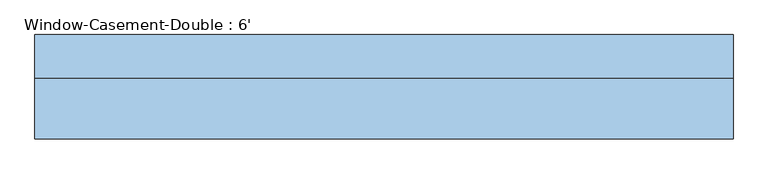
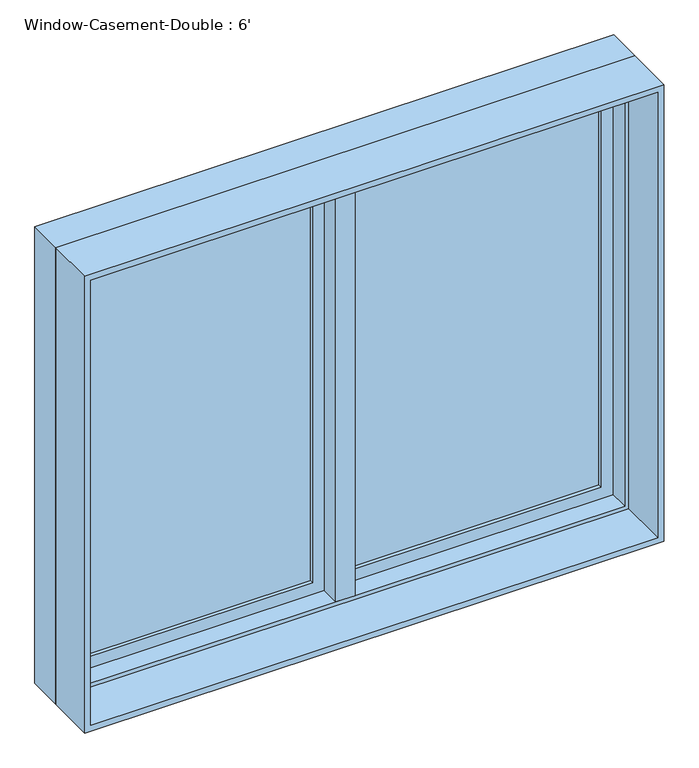
"""IFC4 building model written with IfcOpenShell, lengths in millimetres: window geometry, Window-Casement-Double : 6'."""

from ifc_helpers import new_model, si_unit, frame, origin, place, context, project, spatial, polyline, outline, extrude, faceted_brep, source, transform, mapped, element, save


def window_casement_double_6_75db422f(model_context):
    return source(origin(), model_context, "Body", "SolidModel", [
        faceted_brep([(9.525, 146.05, 2425.7), (-9.525, 146.05, 2425.7), (-9.525, 95.25, 2425.7), (9.525, 95.25, 2425.7), (9.525, 146.05, 927.1), (9.525, 95.25, 927.1), (-9.525, 95.25, 927.1), (-9.525, 146.05, 927.1), (-9.525, 95.25, 946.15), (-9.525, 95.25, 2406.65), (-30.1625, 95.25, 946.15), (-30.1625, 95.25, 2406.65), (-30.1625, 31.75, 946.15), (-30.1625, 31.75, 2406.65), (30.1625, 31.75, 946.15), (30.1625, 31.75, 2406.65), (30.1625, 95.25, 946.15), (30.1625, 95.25, 2406.65), (9.525, 95.25, 946.15), (9.525, 95.25, 2406.65)], [[[0, 1, 2, 3]], [[4, 5, 6, 7]], [[1, 0, 4, 7]], [[2, 1, 7, 6, 8, 9]], [[9, 8, 10, 11]], [[11, 10, 12, 13]], [[13, 12, 14, 15]], [[15, 14, 16, 17]], [[17, 16, 18, 19]], [[0, 3, 19, 18, 5, 4]], [[18, 8, 6, 5]], [[9, 19, 3, 2]], [[8, 18, 16, 14, 12, 10]], [[19, 9, 11, 13, 15, 17]]]),
        extrude(outline(polyline([(-66.675, 127.0), (-66.675, 120.65), (-844.55, 120.65), (-844.55, 127.0), (-66.675, 127.0)])), frame((0.0, 0.0, 984.25), z_axis=(0.0, 0.0, 1.0), x_axis=(1.0, 0.0, 0.0)), (0.0, 0.0, 1.0), 1384.3),
        extrude(outline(polyline([(-844.55, 107.95), (-844.55, 114.3), (-66.675, 114.3), (-66.675, 107.95), (-844.55, 107.95)])), frame((0.0, 0.0, 984.25), z_axis=(0.0, 0.0, 1.0), x_axis=(1.0, 0.0, 0.0)), (0.0, 0.0, 1.0), 1384.3),
        extrude(outline(polyline([(844.55, 127.0), (844.55, 120.65), (66.675, 120.65), (66.675, 127.0), (844.55, 127.0)])), frame((0.0, 0.0, 984.25), z_axis=(0.0, 0.0, 1.0), x_axis=(1.0, 0.0, 0.0)), (0.0, 0.0, 1.0), 1384.3),
        extrude(outline(polyline([(66.675, 107.95), (66.675, 114.3), (844.55, 114.3), (844.55, 107.95), (66.675, 107.95)])), frame((0.0, 0.0, 984.25), z_axis=(0.0, 0.0, 1.0), x_axis=(1.0, 0.0, 0.0)), (0.0, 0.0, 1.0), 1384.3),
        extrude(outline(polyline([(2425.7, -901.7), (927.1, -901.7), (927.1, -9.525), (2425.7, -9.525), (2425.7, -901.7)]), holes=[polyline([(2368.55, -66.675), (984.25, -66.675), (984.25, -844.55), (2368.55, -844.55), (2368.55, -66.675)])]), frame((0.0, 95.25, 0.0), z_axis=(0.0, 1.0, 0.0), x_axis=(0.0, 0.0, 1.0)), (0.0, 0.0, 1.0), 44.45),
        extrude(outline(polyline([(927.1, 901.7), (2425.7, 901.7), (2425.7, 9.525), (927.1, 9.525), (927.1, 901.7)]), holes=[polyline([(984.25, 66.675), (2368.55, 66.675), (2368.55, 844.55), (984.25, 844.55), (984.25, 66.675)])]), frame((0.0, 95.25, 0.0), z_axis=(0.0, 1.0, 0.0), x_axis=(0.0, 0.0, 1.0)), (0.0, 0.0, 1.0), 44.45),
        extrude(outline(polyline([(2438.4, -914.4), (914.4, -914.4), (914.4, 914.4), (2438.4, 914.4), (2438.4, -914.4)]), holes=[polyline([(2419.35, 895.35), (933.45, 895.35), (933.45, -895.35), (2419.35, -895.35), (2419.35, 895.35)])]), frame((0.0, -127.0, 0.0), z_axis=(0.0, 1.0, 0.0), x_axis=(0.0, 0.0, 1.0)), (0.0, 0.0, 1.0), 158.75),
        faceted_brep([(882.65, 95.25, 2406.65), (882.65, 31.75, 2406.65), (-882.65, 31.75, 2406.65), (-882.65, 95.25, 2406.65), (901.7, 146.05, 2425.7), (901.7, 95.25, 2425.7), (-901.7, 95.25, 2425.7), (-901.7, 146.05, 2425.7), (914.4, 31.75, 2438.4), (914.4, 146.05, 2438.4), (-914.4, 146.05, 2438.4), (-914.4, 31.75, 2438.4), (-882.65, 31.75, 946.15), (-882.65, 95.25, 946.15), (-901.7, 95.25, 927.1), (-901.7, 146.05, 927.1), (-914.4, 146.05, 914.4), (-914.4, 31.75, 914.4), (882.65, 31.75, 946.15), (882.65, 95.25, 946.15), (901.7, 95.25, 927.1), (901.7, 146.05, 927.1), (914.4, 146.05, 914.4), (914.4, 31.75, 914.4)], [[[0, 1, 2, 3]], [[4, 5, 6, 7]], [[8, 9, 10, 11]], [[3, 2, 12, 13]], [[7, 6, 14, 15]], [[11, 10, 16, 17]], [[13, 12, 18, 19]], [[15, 14, 20, 21]], [[17, 16, 22, 23]], [[11, 17, 23, 8], [1, 18, 12, 2]], [[19, 18, 1, 0]], [[5, 20, 14, 6], [3, 13, 19, 0]], [[21, 20, 5, 4]], [[23, 22, 9, 8]], [[9, 22, 16, 10], [7, 15, 21, 4]]]),
    ])


if __name__ == "__main__":
    model = new_model("IFC4")
    model_context = context("Model", 3, world=origin())
    ifc_project = project(units=[si_unit("LENGTHUNIT", "METRE", prefix="MILLI")], contexts=[model_context])
    site = spatial("IfcSite", under=ifc_project)
    building = spatial("IfcBuilding", under=site)
    placement = place(None, origin())
    window_casement_double_6_shape = window_casement_double_6_75db422f(model_context)
    element("IfcWindow", 1, ObjectType="Window-Casement-Double : 6'", at=placement, inside=building, context=model_context, shape_type="MappedRepresentation", body=[
        mapped(window_casement_double_6_shape, transform((0.0, 0.0, 0.0), x_axis=(1.0, 0.0, 0.0), y_axis=(0.0, 1.0, 0.0), z_axis=(0.0, 0.0, 1.0))),
    ])
    save(model, "model.ifc")

# Revit data of these elements
# Type "Window-Casement-Double : 6'"
#   Type Mark = "20"
#   Fire Rating = "0.5h"
#   Assembly Code = "B2020100"
#   Analytic Construction = "Double glazing - domestic"
#   Frame Extension [instance default] = 0' - 0 1/4"
#   Window Inset [instance default] = 0' - 0"
#   Wall Thickness [instance default] = 0' - 6"
#   Interior Wall Closure [instance default] = 0' - 2 1/4"
#   Half Width = 3' - 0"
#   Visual Light Transmittance = 0.81
#   Thermal Resistance (R) = 1.8146 (h·ft²·°F)/BTU
#   Solar Heat Gain Coefficient = 0.76
#   Rough Width = 6' - 0 1/2"
#   Rough Height = 5' - 0 1/2"
#   Height = 5' - 0"
#   Heat Transfer Coefficient (U) = 0.5511 BTU/(h·ft²·°F)
#   Exterior Wall Closure [instance default] = 0' - 1 1/4"
#   Extension Jamb [instance default] = 0' - 2 1/4"
#   Default Sill Height = 3' - 0"
#   Width = 6' - 0"
#   Muntin Visibility = yes
#   Interior Trim Visibility [instance default] = yes
#   Exterior Trim Visibility [instance default] = yes
#   Extension Jamb Visibility [instance default] = yes
#   Interior Trim Material = Wood - Stained
#   Muntin Pattern = Muntin Pattern_2x2 : Muntin Pattern_2x2
#   Interior Trim = Trim-Window-Interior-Flat : Picture Frame
#   Interior Frame Material = Wood - Stained
#   Glass Panel Material = Glass
#   Exterior Trim Material = Clad - White
#   Exterior Trim = Trim-Window-Exterior-Flat : with Sill
#   Exterior Frame Material = Clad - White
#   Wall Closure = (empty or 0)
# Element 1 (IfcWindow, "Window-Casement-Double : 6'")
#   Wall Thickness = 0' - 10"
#   Extension Jamb = 0' - 6 1/4"
#   Materials on its faces: "Wood - Stained", "Glass", "Clad - White"
# Materials
#   "Wood - Stained": class "Wood", colour RGB 224 178 126, transparency 0, Cost = 0
#   "Glass": class "Glass", colour RGB 0 128 192, transparency 0.75, Description = "Soda Lime Glass", Cost = 0
#   "Clad - White": class "Wood", colour RGB 242 242 238, transparency 0, Cost = 0
